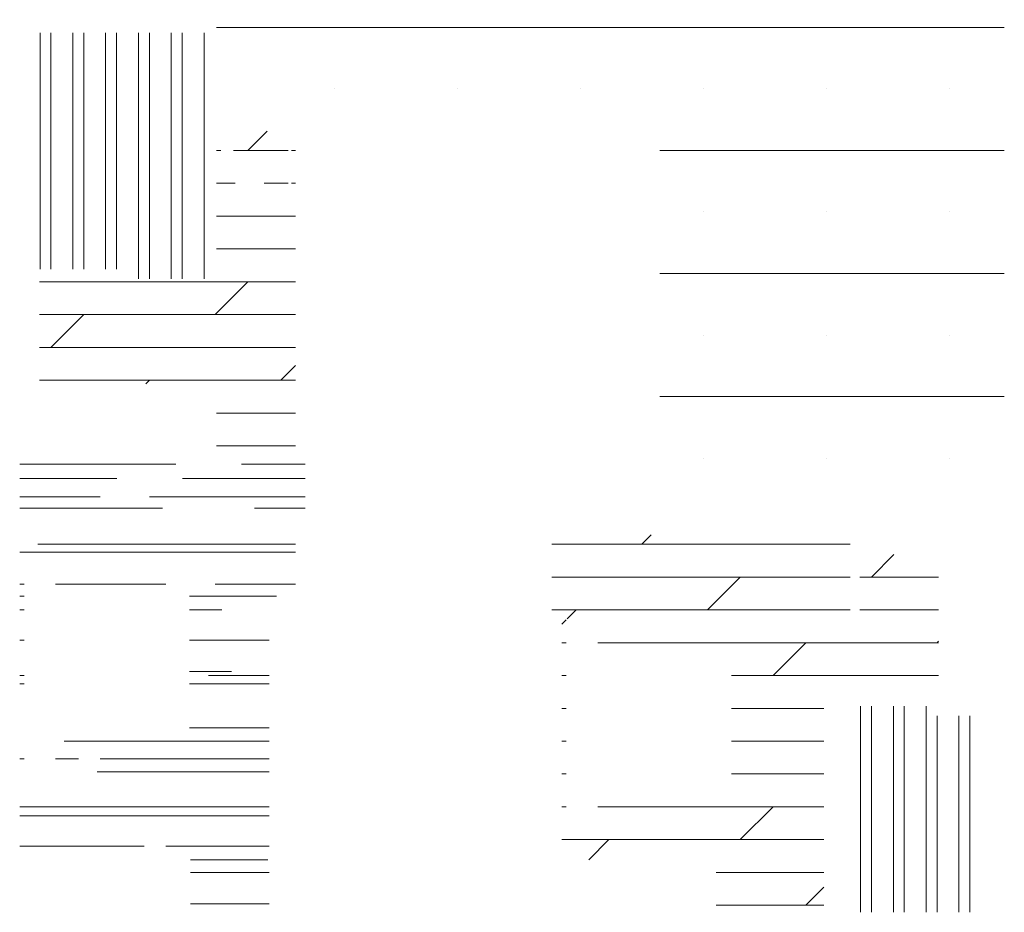
# Model space of a CAD drawing. Units: inches. Extents: x 111008 to 118198, y -138546 to -137723.
# Tile 2 of 4: x 115345 to 115795, y -138452 to -138044. Entities that reach past the tile are written whole.
import ezdxf

# ---------------------------------------------------------------- set-up
doc = ezdxf.new("R2010")
doc.units = ezdxf.units.IN
doc.header["$LTSCALE"] = 20
doc.header["$MEASUREMENT"] = 0
doc.layers.add('A-FLOR-PATT', color=251, linetype='Continuous', lineweight=9)
pattern_1 = [(180, (3579.743, 46.513), (-1e-14, -56.25), []), (180, (3551.62, 74.64), (-1e-14, -56.25), [0, -56.25])]
pattern_2 = [(0, (3579.743, 46.513), (0, 15), []), (45, (3579.743, 46.513), (-30, 30), [21.213203, -42.426407])]
pattern_3 = [(270, (3579.743, 46.513), (15, -9e-16), []), (270, (3574.743, 41.513), (15, -9e-16), [])]

msp = doc.modelspace()

# ---------------------------------------------------------------- hatches: boundary and pattern name
at = {"layer": 'A-FLOR-PATT'}
h = msp.add_hatch(dxfattribs=at)
h.set_pattern_fill('SACNCR', color=256, scale=600, angle=135)
h.set_pattern_definition(pattern_1)
h.paths.add_polyline_path([(115795.46, -138043.69), (115435.46, -138043.69), (115435.46, -138094.69), (115471.46, -138094.69), (115604.96, -138094.69), (115628.96, -138094.69), (115637.96, -138094.69), (115795.46, -138094.69)])
at = {"layer": 'A-FLOR-PATT', "ltscale": 0.5}
h = msp.add_hatch(dxfattribs=at)
h.set_pattern_fill('ANSI32', color=256, scale=40, angle=-135)
h.set_pattern_definition(pattern_3)
h.paths.add_polyline_path([(115430.96, -138049.69), (115345.46, -138049.69), (115345.46, -138085.69), (115345.46, -138157.69), (115397.96, -138157.69), (115397.96, -138162.19), (115430.96, -138162.19)])
at = {"layer": 'A-FLOR-PATT'}
h = msp.add_hatch(dxfattribs=at)
h.set_pattern_fill('DOLMIT', color=256, scale=60)
h.set_pattern_definition(pattern_2)
h.paths.add_polyline_path([(115471.46, -138162.19), (115354.46, -138162.19), (115354.46, -138210.13), (115435.46, -138210.13), (115435.46, -138234.19), (115435.46, -138238.69), (115471.46, -138238.69)])
h.paths.add_polyline_path([(115471.46, -138094.67), (115435.46, -138094.67), (115435.46, -138162.19), (115471.46, -138162.19)])
edge = h.paths.add_edge_path(flags=17)
edge.add_line((115435.46, -138094.69), (115471.46, -138094.69))
h.paths.add_polyline_path([(115469.72, -138130.19), (115469.72, -138097.18), (115468.23, -138097.18), (115468.23, -138130.19)], flags=16)
edge = h.paths.add_edge_path(flags=16)
edge.add_line((115469.03, -138094.69), (115471.46, -138094.69))
edge.add_line((115471.46, -138094.69), (115471.46, -138098.67))
edge.add_line((115471.46, -138098.67), (115469.72, -138098.67))
edge.add_line((115469.72, -138098.67), (115469.72, -138097.18))
edge.add_line((115469.72, -138097.18), (115468.48, -138097.18))
edge.add_line((115468.48, -138097.18), (115468.48, -138095.24))
edge.add_line((115468.48, -138095.24), (115468.62, -138095.24))
edge.add_line((115468.62, -138095.24), (115468.62, -138095.1))
edge.add_arc((115468.89, -138095.1), 0.275, 90, 180, ccw=False)
edge.add_line((115468.89, -138094.83), (115469.03, -138094.83))
edge.add_line((115469.03, -138094.83), (115469.03, -138094.69))
edge = h.paths.add_edge_path(flags=16)
edge.add_line((115437.9, -138094.69), (115435.46, -138094.69))
edge.add_line((115435.46, -138094.69), (115435.46, -138098.67))
edge.add_line((115435.46, -138098.67), (115437.2, -138098.67))
edge.add_line((115437.2, -138098.67), (115437.2, -138097.18))
edge.add_line((115437.2, -138097.18), (115438.45, -138097.18))
edge.add_line((115438.45, -138097.18), (115438.45, -138095.24))
edge.add_line((115438.45, -138095.24), (115438.31, -138095.24))
edge.add_line((115438.31, -138095.24), (115438.31, -138095.1))
edge.add_arc((115438.03, -138095.1), 0.275, 0, 90)
edge.add_line((115438.03, -138094.83), (115437.9, -138094.83))
edge.add_line((115437.9, -138094.83), (115437.9, -138094.69))
edge = h.paths.add_edge_path(flags=16)
edge.add_arc((115468.26, -138099.07), 31.12, 176.5003, 269.9437)
h = msp.add_hatch(dxfattribs=at)
h.set_pattern_fill('SACNCR', color=256, scale=600, angle=135)
h.set_pattern_definition(pattern_1)
h.paths.add_polyline_path([(115795.46, -138094.69), (115637.96, -138094.69), (115637.96, -138111.23), (115637.96, -138159.15), (115637.96, -138210.19), (115637.94, -138270.19), (115795.46, -138270.19)])
h = msp.add_hatch(dxfattribs=at)
h.set_pattern_fill('AR-RROOF', color=256, scale=30, angle=180)
h.set_pattern_definition([(180, (3579.743, 46.513), (-66, -30), [450, -60, 150, -30]), (180, (3539.843, 31.513), (30, -39.9), [90, -9.9, 180, -22.5]), (180, (3564.743, 21.013), (-156, -20.1), [240, -42, 120, -30])])
h.paths.add_polyline_path([(115471.46, -138274.69), (115475.96, -138274.69), (115475.96, -138238.69), (115471.46, -138238.69), (115435.46, -138238.69), (115345.46, -138238.69), (115345.46, -138274.69), (115345.46, -138427.63), (115423.46, -138427.63), (115423.46, -138451.69), (115459.46, -138451.69), (115459.46, -138312.52, -0.414214), (115465.46, -138306.52), (115471.46, -138306.52)])
h.paths.add_polyline_path([(115423.06, -138306.82), (115423.06, -138371.56), (115361.89, -138371.56), (115361.89, -138388.51), (115347.46, -138388.51), (115347.46, -138371.56), (115347.46, -138306.82), (115347.46, -138289.87), (115361.89, -138289.87), (115361.89, -138306.82)], flags=16)
edge = h.paths.add_edge_path(flags=0)
edge.add_line((115421.24, -138308.56), (115421.24, -138369.78))
edge.add_line((115421.24, -138369.78), (115377.84, -138369.78))
edge.add_ellipse((115391.43, -138377.01), major_axis=(-0.72, 20.39), ratio=0.705545, start_angle=59.9505, end_angle=60.0685)
edge.add_line((115377.83, -138369.81), (115377.83, -138369.78))
edge.add_line((115377.83, -138369.78), (115348.19, -138369.78))
edge.add_line((115348.19, -138369.78), (115348.19, -138308.56))
edge.add_line((115348.19, -138308.56), (115421.24, -138308.56))
h.paths.add_polyline_path([(115440.46, -138241.92), (115473.48, -138241.92), (115473.48, -138240.43), (115440.46, -138240.43)], flags=16)
h.paths.add_polyline_path([(115365.48, -138365.92), (115351.85, -138365.92), (115351.85, -138341.73), (115365.48, -138341.73), (115365.48, -138337.96), (115351.85, -138337.96), (115351.85, -138313.77), (115365.48, -138313.77)], flags=0)
h = msp.add_hatch(dxfattribs=at)
h.set_pattern_fill('DOLMIT', color=256, scale=60)
h.set_pattern_definition(pattern_2)
h.paths.add_polyline_path([(115724.96, -138279.19), (115588.71, -138279.19), (115588.71, -138315.21), (115593.21, -138315.21), (115593.21, -138427.63), (115663.71, -138427.63), (115663.71, -138451.69), (115712.96, -138451.69), (115712.96, -138351.21, -0.414214), (115715.96, -138348.21), (115724.96, -138348.21), (115724.96, -138315.21)])
h.paths.add_polyline_path([(115670.81, -138334.65), (115670.81, -138399.38), (115609.64, -138399.38), (115609.64, -138414.77), (115595.21, -138414.77), (115595.21, -138399.38), (115595.21, -138334.65), (115595.21, -138317.52), (115609.64, -138317.52), (115609.64, -138334.65)], flags=16)
edge = h.paths.add_edge_path(flags=0)
edge.add_line((115668.98, -138336.39), (115668.98, -138397.61))
edge.add_line((115668.98, -138397.61), (115625.58, -138397.61))
edge.add_ellipse((115639.17, -138404.84), major_axis=(-0.72, 20.39), ratio=0.705545, start_angle=59.9505, end_angle=60.0685)
edge.add_line((115625.58, -138397.64), (115625.57, -138397.61))
edge.add_line((115625.57, -138397.61), (115595.94, -138397.61))
edge.add_line((115595.94, -138397.61), (115595.94, -138336.39))
edge.add_line((115595.94, -138336.39), (115668.98, -138336.39))
h.paths.add_polyline_path([(115624.21, -138282.42), (115591.19, -138282.42), (115591.19, -138280.93), (115624.21, -138280.93)], flags=16)
h.paths.add_polyline_path([(115613.22, -138393.74), (115599.59, -138393.74), (115599.59, -138369.56), (115613.22, -138369.56), (115613.22, -138365.79), (115599.59, -138365.79), (115599.59, -138341.6), (115613.22, -138341.6)], flags=0)
h = msp.add_hatch(dxfattribs=at)
h.set_pattern_fill('DOLMIT', color=256, scale=60)
h.set_pattern_definition(pattern_2)
h.paths.add_polyline_path([(115765.4, -138288.19), (115729.46, -138288.19), (115729.46, -138315.21), (115724.96, -138315.21), (115724.96, -138348.21), (115729.46, -138348.21), (115729.46, -138357.44), (115765.4, -138357.44)])
at = {"layer": 'A-FLOR-PATT', "ltscale": 0.5}
h = msp.add_hatch(dxfattribs=at)
h.set_pattern_fill('ANSI32', color=256, scale=40, angle=-135)
h.set_pattern_definition(pattern_3)
h.paths.add_polyline_path([(115789.46, -138361.94), (115762.46, -138361.94), (115762.46, -138357.44), (115729.46, -138357.44), (115729.46, -138451.69), (115789.46, -138451.69)])

doc.saveas('drawing.dxf')
